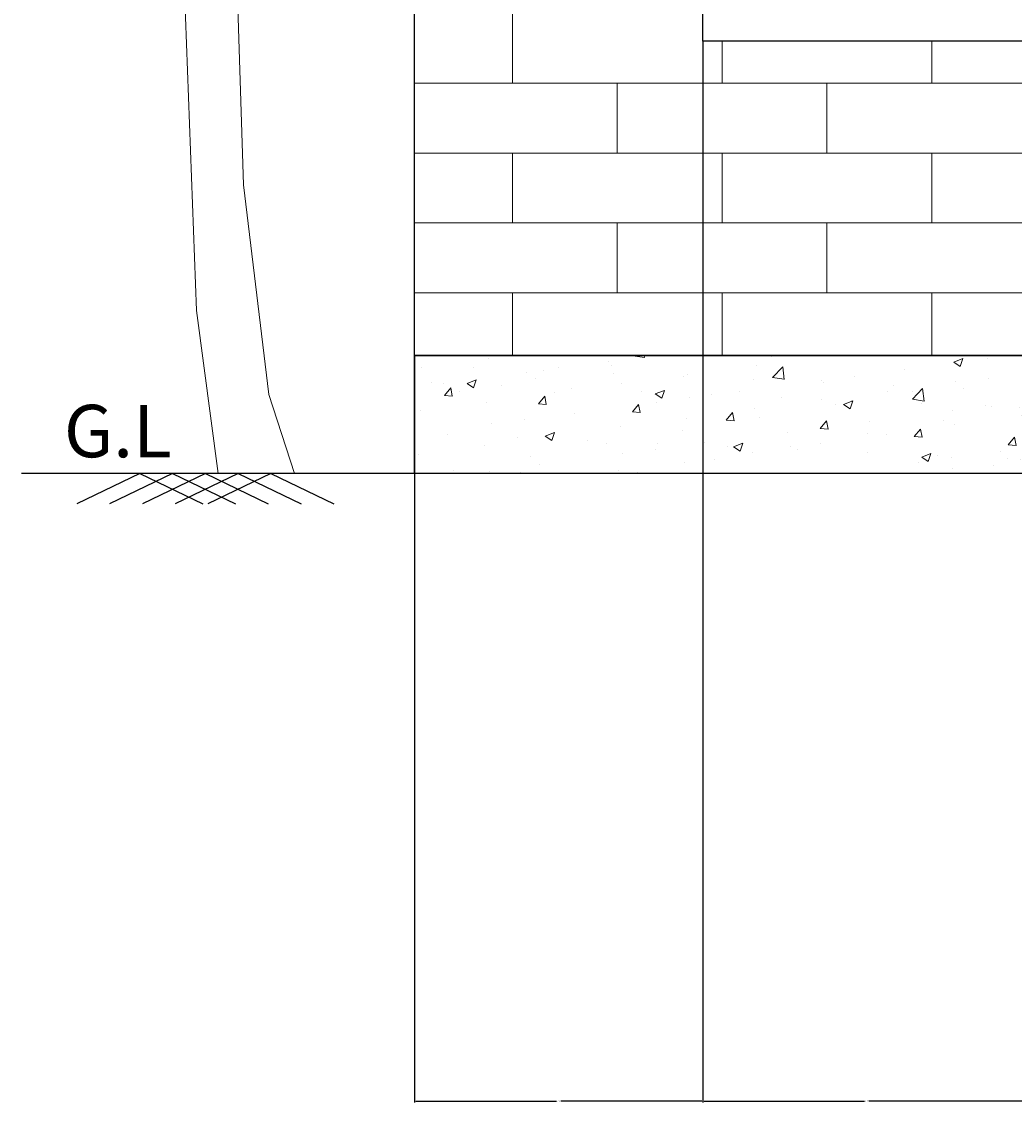
# Model space of a CAD drawing. Units: inches. Extents: x 37 to 824, y -700 to 234.
# Tile 1 of 77: x 101 to 253, y -700 to -535. Entities that reach past the tile are written whole.
import ezdxf

# ---------------------------------------------------------------- set-up
doc = ezdxf.new("R2010")
doc.units = ezdxf.units.IN
doc.header["$MEASUREMENT"] = 0
for name, color, linetype, lineweight in [('A-ANNO-DIMS', 2, 'Continuous', 18), ('A-ANNO-TEXT', 7, 'Continuous', 18), ('A-ELEV', 3, 'Continuous', 25), ('A-ELEV-PATT', 8, 'Continuous', 13), ('A-SITE-PLNT', 3, 'Continuous', 13)]:
    doc.layers.add(name, color=color, linetype=linetype, lineweight=lineweight)
doc.styles.get("Standard").update_dxf_attribs({"font": 'arial.ttf'})
doc.dimstyles.get("Standard").update_dxf_attribs({"dimtxt": 0.18, "dimasz": 0.18, "dimexe": 0.18, "dimexo": 0.0625, "dimgap": 0.09, "dimtad": 0, "dimtih": 1, "dimtoh": 1, "dimdec": 1, "dimzin": 0, "dimdsep": 46, "dimlunit": 4, "dimtxsty": 'Standard', "dimcen": 0.09, "dimadec": 0, "dimazin": 0, "dimtfac": 1, "dimtdec": 1, "dimtofl": 0, "dimtmove": 0, "dimatfit": 3, "dimfxl": 1, "dimtolj": 1, "dimtzin": 0, "dimarcsym": 0})

# ---------------------------------------------------------------- blocks, each defined once
blk = doc.blocks.new('*U34')
for points in [[(-2.363, 170.553), (-3.88, 148.505), (-4.988, 69.634), (-3.325, 24.869), (0, 0)], [(-0.116, 162.848), (0.554, 143.532), (2.217, 96.635), (3.88, 44.054), (7.76, 12.079), (11.64, 0)]]:
    blk.add_lwpolyline(points)
blk = doc.blocks.new('*D67')
at = {"layer": 'A-ANNO-DIMS', "color": 0, "lineweight": -2, "ltscale": 0.5, "transparency": 16777216}
for p, q in [((205.08, -537.69), (205.08, -699.59)), ((161.08, -585.69), (161.08, -699.59)), ((161.26, -699.41), (182.75, -699.41)), ((204.9, -699.41), (183.41, -699.41))]:
    blk.add_line(p, q, dxfattribs=at)
at = {"layer": 'A-ANNO-DIMS', "color": 0, "ltscale": 0.5, "transparency": 16777216}
for points in [[(161.26, -699.38), (161.26, -699.44), (161.08, -699.41)], [(204.9, -699.38), (204.9, -699.44), (205.08, -699.41)]]:
    blk.add_solid(points, dxfattribs=at)
at = {"layer": 'Defpoints', "color": 0, "ltscale": 0.5, "transparency": 16777216}
for p in [(205.08, -537.63), (161.08, -585.63), (205.08, -699.41)]:
    blk.add_point(p, dxfattribs=at)
at = {"layer": 'A-ANNO-DIMS', "color": 0, "ltscale": 0.5, "transparency": 16777216, "insert": (183.08, -699.41), "char_height": 0.18, "attachment_point": 5}
blk.add_mtext('\\A1;3\'-8"', dxfattribs=at)
blk = doc.blocks.new('*D68')
at = {"layer": 'A-ANNO-DIMS', "color": 0, "lineweight": -2, "ltscale": 0.5, "transparency": 16777216}
for p, q in [((205.08, -537.69), (205.08, -699.59)), ((255.08, -537.69), (255.08, -699.59)), ((205.26, -699.41), (229.74, -699.41)), ((254.9, -699.41), (230.41, -699.41))]:
    blk.add_line(p, q, dxfattribs=at)
at = {"layer": 'A-ANNO-DIMS', "color": 0, "ltscale": 0.5, "transparency": 16777216}
for points in [[(205.26, -699.38), (205.26, -699.44), (205.08, -699.41)], [(254.9, -699.38), (254.9, -699.44), (255.08, -699.41)]]:
    blk.add_solid(points, dxfattribs=at)
at = {"layer": 'Defpoints', "color": 0, "ltscale": 0.5, "transparency": 16777216}
for p in [(205.08, -537.63), (255.08, -537.63), (255.08, -699.41)]:
    blk.add_point(p, dxfattribs=at)
at = {"layer": 'A-ANNO-DIMS', "color": 0, "ltscale": 0.5, "transparency": 16777216, "insert": (230.08, -699.41), "char_height": 0.18, "attachment_point": 5}
blk.add_mtext('\\A1;4\'-2"', dxfattribs=at)

msp = doc.modelspace()

# ---------------------------------------------------------------- hatches: boundary and pattern name
at = {"layer": 'A-ELEV-PATT', "ltscale": 0.5}
h = msp.add_hatch(dxfattribs=at)
h.set_pattern_fill('AR-BRSTD', color=256, scale=4)
h.paths.add_polyline_path([(299.08, -489.63), (358.13, -489.63), (358.13, -585.63), (428.08, -585.63), (428.08, -465.63), (161.08, -465.63), (161.08, -585.63), (299.08, -585.63)])
h.paths.add_polyline_path([(205.08, -537.63), (205.08, -489.63), (255.08, -489.63), (255.08, -537.63)], flags=16)
h = msp.add_hatch(dxfattribs=at)
h.set_pattern_fill('AR-CONC', color=256, scale=2)
h.paths.add_polyline_path([(299.08, -585.63), (161.08, -585.63), (161.08, -603.63), (299.08, -603.63)])
h.paths.add_polyline_path([(428.08, -585.63), (358.13, -585.63), (358.13, -603.63), (428.08, -603.63)])

# ---------------------------------------------------------------- linework, layer by layer
at = {"layer": 'A-ELEV', "ltscale": 0.5}
for p, q in [((161.08, -603.63), (101.08, -603.63)), ((119.13, -603.63), (109.52, -608.24)), ((124.13, -603.63), (114.52, -608.24)), ((119.13, -603.63), (128.74, -608.24)), ((129.13, -603.63), (119.52, -608.24)), ((124.13, -603.63), (133.74, -608.24)), ((134.13, -603.63), (124.52, -608.24)), ((129.13, -603.63), (138.74, -608.24)), ((139.13, -603.63), (129.52, -608.24)), ((134.13, -603.63), (143.74, -608.24)), ((139.13, -603.63), (148.74, -608.24))]:
    msp.add_line(p, q, dxfattribs=at)
for points in [[(161.08, -465.63), (428.08, -465.63), (428.08, -585.63), (161.08, -585.63)], [(205.08, -489.63), (255.08, -489.63), (255.08, -537.63), (205.08, -537.63)], [(161.08, -585.63), (428.08, -585.63), (428.08, -603.63), (161.08, -603.63)]]:
    msp.add_lwpolyline(points, close=True, dxfattribs=at)

# ---------------------------------------------------------------- block references
at = {"layer": 'A-SITE-PLNT'}
msp.add_blockref('*U34', (131.08, -603.63), dxfattribs=at)

# ---------------------------------------------------------------- texts
at = {"layer": 'A-ANNO-TEXT'}
msp.add_text('G.L', height=8, dxfattribs=at).set_placement((107.54, -601.15))

# ---------------------------------------------------------------- dimensions: what is measured, and where the dimension line sits
at = {"layer": 'A-ANNO-DIMS', "ltscale": 0.5}
for base, p1, p2, picture, middle in [((205.08, -699.41), (161.08, -585.63), (205.08, -537.63), '*D67', (183.08, -699.41)), ((255.08, -699.41), (205.08, -537.63), (255.08, -537.63), '*D68', (230.08, -699.41))]:
    dim = msp.add_linear_dim(base=base, p1=p1, p2=p2, dimstyle='Standard', override={"dimdec": 1, "dimlfac": 1, "dimrnd": 0, "dimzin": 1, "dimdsep": 46, "dimlunit": 4, "dimfrac": 2}, dxfattribs=at)
    dim.commit()
    dim.dimension.update_dxf_attribs({"geometry": picture, "text_midpoint": middle})

doc.saveas('drawing.dxf')
